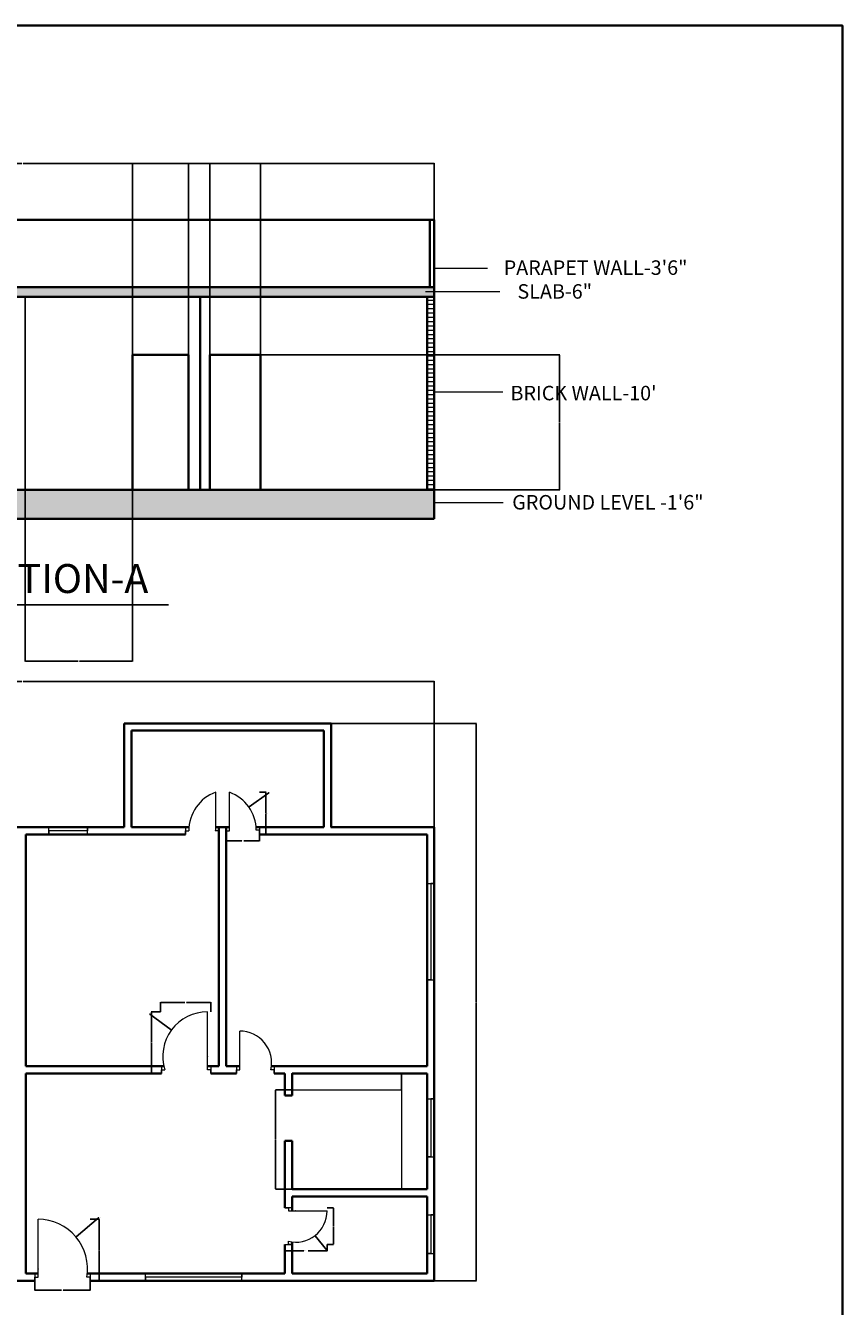
# Model space of a CAD drawing. Units: inches. Extents: x 2055 to 3558, y 1520 to 2888.
# Tile 8 of 8: x 3050 to 3558, y 2092 to 2888. Entities that reach past the tile are written whole.
import ezdxf

# ---------------------------------------------------------------- set-up
doc = ezdxf.new("R2010")
doc.units = ezdxf.units.IN
for name, color, linetype, lineweight in [('A-ANNO-DIMS', 2, 'Continuous', 18), ('A-ANNO-TEXT', 7, 'Continuous', 18), ('A-ANNO-TTLB', 7, 'Continuous', 35), ('A-DOOR', 3, 'Continuous', 18), ('A-FLOR-FIXT', 8, 'Continuous', 18), ('A-GLAZ', 4, 'Continuous', 18), ('A-SECT', 7, 'Continuous', 35), ('A-SECT-PATT', 252, 'Continuous', 13), ('A-WALL', 7, 'Continuous', 35), ('A-WALL-PATT', 252, 'Continuous', 13)]:
    doc.layers.add(name, color=color, linetype=linetype, lineweight=lineweight)
doc.styles.get("Standard").update_dxf_attribs({"font": 'arial.ttf'})
doc.dimstyles.get("Standard").update_dxf_attribs({"dimtxt": 0.18, "dimasz": 0.18, "dimexe": 0.18, "dimexo": 0.0625, "dimgap": 0.09, "dimtad": 0, "dimtih": 1, "dimtoh": 1, "dimdec": 4, "dimzin": 0, "dimdsep": 46, "dimtxsty": 'Standard', "dimcen": 0.09, "dimadec": 0, "dimazin": 0, "dimtfac": 1, "dimtdec": 4, "dimtofl": 0, "dimtmove": 0, "dimatfit": 3, "dimfxl": 1, "dimtolj": 1, "dimtzin": 0, "dimarcsym": 0})

# ---------------------------------------------------------------- blocks, each defined once
blk = doc.blocks.new('DOOR-BED-36-C')
for p, q in [((28.6, 2.25), (28.6, 38.25)), ((0, 4.5), (0, 0)), ((0, 0), (0, 2.25)), ((0, 2.25), (2, 2.25)), ((30.6, 2.25), (28.6, 2.25)), ((30.6, 4.5), (30.6, 0)), ((30.6, 0), (30.6, 2.25))]:
    blk.add_line(p, q)
blk.add_arc((28.6, 10.43), 27.83, 90, 197.08497)
blk = doc.blocks.new('DOOR-BED-24-A')
for p, q in [((2, 2.25), (2, 26.25)), ((0, 4.5), (0, 0)), ((0, 0), (0, 2.25)), ((0, 2.25), (2, 2.25)), ((23.39, 2.25), (21.39, 2.25)), ((23.39, 4.5), (23.39, 0)), ((23.39, 0), (23.39, 2.25))]:
    blk.add_line(p, q)
blk.add_arc((2, 6.42), 19.83, 347.8769, 90)
blk = doc.blocks.new('DOOR-BATH-24-A')
for p, q in [((4.5, 22.87), (0, 22.87)), ((0, 22.87), (2.25, 22.87)), ((2.25, 22.87), (2.25, 20.87)), ((2.25, 20.87), (26.25, 20.87)), ((2.25, 0), (2.25, 2)), ((0, 0), (4.5, 0)), ((4.5, 0), (2.25, 0))]:
    blk.add_line(p, q)
blk.add_arc((6.83, 20.87), 19.42, 256.35438, 0)
blk = doc.blocks.new('DOOR-ENTRY-36-A')
for p, q in [((2, 2.25), (2, 38.25)), ((0, 4.5), (0, 0)), ((0, 0), (0, 2.25)), ((0, 2.25), (2, 2.25)), ((34.35, 2.25), (32.35, 2.25)), ((34.35, 4.5), (34.35, 0)), ((34.35, 0), (34.35, 2.25))]:
    blk.add_line(p, q)
blk.add_arc((2, 7.46), 30.8, 350.26968, 90)
blk = doc.blocks.new('DOOR-VERANDA-24-G')
for p, q in [((18.74, 2.29), (18.74, 26.29)), ((0, 4.5), (0, 0)), ((0, 0), (0, 2.25)), ((0, 2.25), (2, 2.25)), ((20.74, 2.29), (18.74, 2.29))]:
    blk.add_line(p, q)
blk.add_arc((27.63, 2.25), 25.63, 110.29699, 180)
blk = doc.blocks.new('DOOR-VERANDA-24-H')
for p, q in [((2, 2.19), (2, 26.19)), ((0, 2.19), (2, 2.19)), ((20.78, 2.69), (18.78, 2.69)), ((20.78, 4.5), (20.78, 0)), ((20.78, 0), (20.78, 2.69))]:
    blk.add_line(p, q)
blk.add_arc((-6.63, 2.38), 25.41, 0.68308, 70.14714)
blk = doc.blocks.new('WIN-36')
for p, q in [((2.25, 36), (0, 36)), ((0, 36), (4.5, 36)), ((2.25, 0), (2.25, 36)), ((0, 0), (4.5, 0)), ((4.5, 0), (2.25, 0))]:
    blk.add_line(p, q)
blk = doc.blocks.new('WIN-24')
for p, q in [((0, 24), (4.5, 24)), ((4.5, 24), (2.25, 24)), ((2.25, 24), (2.25, 0)), ((2.25, 0), (0, 0)), ((0, 0), (4.5, 0))]:
    blk.add_line(p, q)
blk = doc.blocks.new('WIN-60')
for p, q in [((0, 60), (4.5, 60)), ((4.5, 60), (2.25, 60)), ((2.25, 60), (2.25, 0)), ((2.25, 0), (0, 0)), ((0, 0), (4.5, 0))]:
    blk.add_line(p, q)
blk = doc.blocks.new('COUNTER-2')
for p, q in [((0, 61.79), (68.13, 61.79)), ((68.13, 61.79), (68.13, 0))]:
    blk.add_line(p, q)
blk = doc.blocks.new('VERANDA-PERIMETER')
for p, q in [((0, 0), (0, 64.5)), ((4.5, 64.5), (4.5, 4.5)), ((124.15, 4.5), (124.15, 64.5)), ((128.65, 64.5), (128.65, 4.5)), ((4.5, 0), (0, 0)), ((4.5, 4.5), (124.15, 4.5)), ((128.65, 0), (4.5, 0)), ((128.65, 4.5), (128.65, 0))]:
    blk.add_line(p, q)
blk = doc.blocks.new('*D56')
at = {"layer": 'A-ANNO-DIMS', "color": 0, "lineweight": -2, "transparency": 16777216}
for p, q in [((3133.65, 2275.25), (3127.79, 2275.25)), ((3127.97, 2275.07), (3127.97, 2256.31)), ((3127.97, 2237.18), (3127.97, 2255.94)), ((3133.65, 2237), (3127.79, 2237))]:
    blk.add_line(p, q, dxfattribs=at)
at = {"layer": 'A-ANNO-DIMS', "color": 0, "transparency": 16777216}
for points in [[(3127.94, 2275.07), (3128, 2275.07), (3127.97, 2275.25)], [(3127.94, 2237.18), (3128, 2237.18), (3127.97, 2237)]]:
    blk.add_solid(points, dxfattribs=at)
at = {"layer": 'Defpoints', "color": 0, "transparency": 16777216}
for p in [(3127.97, 2275.25), (3133.71, 2275.25), (3133.71, 2237)]:
    blk.add_point(p, dxfattribs=at)
at = {"layer": 'A-ANNO-DIMS', "color": 0, "transparency": 16777216, "insert": (3127.97, 2256.12), "char_height": 0.18, "attachment_point": 5}
blk.add_mtext('\\A1;BED DOOR 38 TYP.', dxfattribs=at)
blk = doc.blocks.new('*D57')
at = {"layer": 'A-ANNO-DIMS', "color": 0, "lineweight": -2, "transparency": 16777216}
for p, q in [((3133.71, 2275.31), (3133.71, 2281.17)), ((3133.89, 2280.99), (3148.78, 2280.99)), ((3164.72, 2280.99), (3149.83, 2280.99)), ((3164.9, 2275.31), (3164.9, 2281.17))]:
    blk.add_line(p, q, dxfattribs=at)
at = {"layer": 'A-ANNO-DIMS', "color": 0, "transparency": 16777216}
for points in [[(3133.89, 2281.02), (3133.89, 2280.96), (3133.71, 2280.99)], [(3164.72, 2281.02), (3164.72, 2280.96), (3164.9, 2280.99)]]:
    blk.add_solid(points, dxfattribs=at)
at = {"layer": 'Defpoints', "color": 0, "transparency": 16777216}
for p in [(3164.9, 2280.99), (3133.71, 2275.25), (3164.9, 2275.25)]:
    blk.add_point(p, dxfattribs=at)
at = {"layer": 'A-ANNO-DIMS', "color": 0, "transparency": 16777216, "insert": (3149.3, 2280.99), "char_height": 0.18, "attachment_point": 5}
blk.add_mtext('\\A1;31 TYP.', dxfattribs=at)
blk = doc.blocks.new('*D60')
at = {"layer": 'A-ANNO-DIMS', "color": 0, "lineweight": -2, "transparency": 16777216}
for p, q in [((3211, 2130.52), (3211, 2126.46)), ((3211.18, 2126.64), (3222.81, 2126.64)), ((3237.07, 2126.64), (3225.43, 2126.64)), ((3237.25, 2130.52), (3237.25, 2126.46))]:
    blk.add_line(p, q, dxfattribs=at)
at = {"layer": 'A-ANNO-DIMS', "color": 0, "transparency": 16777216}
for points in [[(3211.18, 2126.67), (3211.18, 2126.61), (3211, 2126.64)], [(3237.07, 2126.67), (3237.07, 2126.61), (3237.25, 2126.64)]]:
    blk.add_solid(points, dxfattribs=at)
at = {"layer": 'Defpoints', "color": 0, "transparency": 16777216}
for p in [(3211, 2130.58), (3237.25, 2130.58), (3237.25, 2126.64)]:
    blk.add_point(p, dxfattribs=at)
at = {"layer": 'A-ANNO-DIMS', "color": 0, "transparency": 16777216, "insert": (3224.12, 2126.64), "char_height": 0.18, "attachment_point": 5}
blk.add_mtext('\\A1;BATH DOOR 26 TYP.', dxfattribs=at)
blk = doc.blocks.new('*D61')
at = {"layer": 'A-ANNO-DIMS', "color": 0, "lineweight": -2, "transparency": 16777216}
for p, q in [((3237.31, 2153.45), (3241.36, 2153.45)), ((3241.18, 2153.27), (3241.18, 2142.2)), ((3241.18, 2130.76), (3241.18, 2141.84)), ((3237.31, 2130.58), (3241.36, 2130.58))]:
    blk.add_line(p, q, dxfattribs=at)
at = {"layer": 'A-ANNO-DIMS', "color": 0, "transparency": 16777216}
for points in [[(3241.15, 2153.27), (3241.21, 2153.27), (3241.18, 2153.45)], [(3241.15, 2130.76), (3241.21, 2130.76), (3241.18, 2130.58)]]:
    blk.add_solid(points, dxfattribs=at)
at = {"layer": 'Defpoints', "color": 0, "transparency": 16777216}
for p in [(3237.25, 2153.45), (3241.18, 2153.45), (3237.25, 2130.58)]:
    blk.add_point(p, dxfattribs=at)
at = {"layer": 'A-ANNO-DIMS', "color": 0, "transparency": 16777216, "insert": (3241.18, 2142.02), "char_height": 0.18, "attachment_point": 5}
blk.add_mtext('\\A1;23 TYP.', dxfattribs=at)
blk = doc.blocks.new('*D62')
at = {"layer": 'A-ANNO-DIMS', "color": 0, "lineweight": -2, "transparency": 16777216}
for p, q in [((3089.92, 2146.25), (3095.78, 2146.25)), ((3095.6, 2146.07), (3095.6, 2127.31)), ((3095.6, 2108.18), (3095.6, 2126.94)), ((3089.92, 2108), (3095.78, 2108))]:
    blk.add_line(p, q, dxfattribs=at)
at = {"layer": 'A-ANNO-DIMS', "color": 0, "transparency": 16777216}
for points in [[(3095.57, 2146.07), (3095.63, 2146.07), (3095.6, 2146.25)], [(3095.57, 2108.18), (3095.63, 2108.18), (3095.6, 2108)]]:
    blk.add_solid(points, dxfattribs=at)
at = {"layer": 'Defpoints', "color": 0, "transparency": 16777216}
for p in [(3089.86, 2146.25), (3095.6, 2146.25), (3089.86, 2108)]:
    blk.add_point(p, dxfattribs=at)
at = {"layer": 'A-ANNO-DIMS', "color": 0, "transparency": 16777216, "insert": (3095.6, 2127.12), "char_height": 0.18, "attachment_point": 5}
blk.add_mtext('\\A1;ENTRY DOOR 38 TYP.', dxfattribs=at)
blk = doc.blocks.new('*D63')
at = {"layer": 'A-ANNO-DIMS', "color": 0, "lineweight": -2, "transparency": 16777216}
for p, q in [((3055.51, 2107.94), (3055.51, 2102.08)), ((3055.69, 2102.26), (3072.16, 2102.26)), ((3089.68, 2102.26), (3073.21, 2102.26)), ((3089.86, 2107.94), (3089.86, 2102.08))]:
    blk.add_line(p, q, dxfattribs=at)
at = {"layer": 'A-ANNO-DIMS', "color": 0, "transparency": 16777216}
for points in [[(3055.69, 2102.29), (3055.69, 2102.23), (3055.51, 2102.26)], [(3089.68, 2102.29), (3089.68, 2102.23), (3089.86, 2102.26)]]:
    blk.add_solid(points, dxfattribs=at)
at = {"layer": 'Defpoints', "color": 0, "transparency": 16777216}
for p in [(3055.51, 2108), (3089.86, 2108), (3089.86, 2102.26)]:
    blk.add_point(p, dxfattribs=at)
at = {"layer": 'A-ANNO-DIMS', "color": 0, "transparency": 16777216, "insert": (3072.69, 2102.26), "char_height": 0.18, "attachment_point": 5}
blk.add_mtext('\\A1;34 TYP.', dxfattribs=at)
blk = doc.blocks.new('*D96')
at = {"layer": 'A-ANNO-DIMS', "color": 0, "lineweight": -2, "transparency": 16777216}
for p, q in [((3195.34, 2411.79), (3199.4, 2411.79)), ((3199.22, 2411.61), (3199.22, 2398.83)), ((3199.22, 2385.68), (3199.22, 2398.46)), ((3195.34, 2385.5), (3199.4, 2385.5))]:
    blk.add_line(p, q, dxfattribs=at)
at = {"layer": 'A-ANNO-DIMS', "color": 0, "transparency": 16777216}
for points in [[(3199.19, 2411.61), (3199.25, 2411.61), (3199.22, 2411.79)], [(3199.19, 2385.68), (3199.25, 2385.68), (3199.22, 2385.5)]]:
    blk.add_solid(points, dxfattribs=at)
at = {"layer": 'Defpoints', "color": 0, "transparency": 16777216}
for p in [(3195.28, 2411.79), (3199.22, 2411.79), (3195.28, 2385.5)]:
    blk.add_point(p, dxfattribs=at)
at = {"layer": 'A-ANNO-DIMS', "color": 0, "transparency": 16777216, "insert": (3199.22, 2398.64), "char_height": 0.18, "attachment_point": 5}
blk.add_mtext('\\A1;VERANDA DOOR 26 TYP.', dxfattribs=at)
blk = doc.blocks.new('*D97')
at = {"layer": 'A-ANNO-DIMS', "color": 0, "lineweight": -2, "transparency": 16777216}
for p, q in [((3174.5, 2385.44), (3174.5, 2381.38)), ((3174.68, 2381.56), (3184.36, 2381.56)), ((3195.1, 2381.56), (3185.42, 2381.56)), ((3195.28, 2385.44), (3195.28, 2381.38))]:
    blk.add_line(p, q, dxfattribs=at)
at = {"layer": 'A-ANNO-DIMS', "color": 0, "transparency": 16777216}
for points in [[(3174.68, 2381.59), (3174.68, 2381.53), (3174.5, 2381.56)], [(3195.1, 2381.59), (3195.1, 2381.53), (3195.28, 2381.56)]]:
    blk.add_solid(points, dxfattribs=at)
at = {"layer": 'Defpoints', "color": 0, "transparency": 16777216}
for p in [(3174.5, 2385.5), (3195.28, 2385.5), (3195.28, 2381.56)]:
    blk.add_point(p, dxfattribs=at)
at = {"layer": 'A-ANNO-DIMS', "color": 0, "transparency": 16777216, "insert": (3184.89, 2381.56), "char_height": 0.18, "attachment_point": 5}
blk.add_mtext('\\A1;21 TYP.', dxfattribs=at)
blk = doc.blocks.new('*D108')
at = {"layer": 'A-ANNO-DIMS', "color": 0, "lineweight": -2, "transparency": 16777216}
for p, q in [((3215.5, 2226.85), (3215.5, 2237.19)), ((3283.62, 2226.85), (3283.62, 2237.19)), ((3215.68, 2237.01), (3248.38, 2237.01)), ((3283.44, 2237.01), (3250.74, 2237.01))]:
    blk.add_line(p, q, dxfattribs=at)
at = {"layer": 'A-ANNO-DIMS', "color": 0, "transparency": 16777216}
for points in [[(3215.68, 2237.04), (3215.68, 2236.98), (3215.5, 2237.01)], [(3283.44, 2237.04), (3283.44, 2236.98), (3283.62, 2237.01)]]:
    blk.add_solid(points, dxfattribs=at)
at = {"layer": 'Defpoints', "color": 0, "transparency": 16777216}
for p in [(3283.62, 2237.01), (3215.5, 2226.79), (3283.62, 2226.79)]:
    blk.add_point(p, dxfattribs=at)
at = {"layer": 'A-ANNO-DIMS', "color": 0, "transparency": 16777216, "insert": (3249.56, 2237.01), "char_height": 0.18, "attachment_point": 5}
blk.add_mtext('\\A1;COUNTER 68 TYP.', dxfattribs=at)
blk = doc.blocks.new('*D109')
at = {"layer": 'A-ANNO-DIMS', "color": 0, "lineweight": -2, "transparency": 16777216}
for p, q in [((3215.43, 2226.79), (3205.1, 2226.79)), ((3205.28, 2226.61), (3205.28, 2196.08)), ((3205.28, 2165.18), (3205.28, 2195.71)), ((3215.43, 2165), (3205.1, 2165))]:
    blk.add_line(p, q, dxfattribs=at)
at = {"layer": 'A-ANNO-DIMS', "color": 0, "transparency": 16777216}
for points in [[(3205.25, 2226.61), (3205.31, 2226.61), (3205.28, 2226.79)], [(3205.25, 2165.18), (3205.31, 2165.18), (3205.28, 2165)]]:
    blk.add_solid(points, dxfattribs=at)
at = {"layer": 'Defpoints', "color": 0, "transparency": 16777216}
for p in [(3205.28, 2226.79), (3215.5, 2226.79), (3215.5, 2165)]:
    blk.add_point(p, dxfattribs=at)
at = {"layer": 'A-ANNO-DIMS', "color": 0, "transparency": 16777216, "insert": (3205.28, 2195.9), "char_height": 0.18, "attachment_point": 5}
blk.add_mtext('\\A1;62 TYP.', dxfattribs=at)
blk = doc.blocks.new('*D124')
at = {"layer": 'A-ANNO-DIMS', "color": 0, "lineweight": -2, "transparency": 16777216}
for p, q in [((2791.5, 2390.06), (2791.5, 2480.78)), ((2791.68, 2480.6), (3047.35, 2480.6)), ((3303.82, 2480.6), (3048.14, 2480.6)), ((3304, 2390.06), (3304, 2480.78))]:
    blk.add_line(p, q, dxfattribs=at)
at = {"layer": 'A-ANNO-DIMS', "color": 0, "transparency": 16777216}
for points in [[(2791.68, 2480.63), (2791.68, 2480.57), (2791.5, 2480.6)], [(3303.82, 2480.63), (3303.82, 2480.57), (3304, 2480.6)]]:
    blk.add_solid(points, dxfattribs=at)
at = {"layer": 'Defpoints', "color": 0, "transparency": 16777216}
for p in [(3304, 2480.6), (2791.5, 2390), (3304, 2390)]:
    blk.add_point(p, dxfattribs=at)
at = {"layer": 'A-ANNO-DIMS', "color": 0, "transparency": 16777216, "insert": (3047.75, 2480.6), "char_height": 0.18, "attachment_point": 5}
blk.add_mtext('\\A1;512.5', dxfattribs=at)
blk = doc.blocks.new('*D125')
at = {"layer": 'A-ANNO-DIMS', "color": 0, "lineweight": -2, "transparency": 16777216}
for p, q in [((3239.79, 2454.5), (3330.28, 2454.5)), ((3330.1, 2454.32), (3330.1, 2281.43)), ((3330.1, 2108.18), (3330.1, 2281.07)), ((3304.06, 2108), (3330.28, 2108))]:
    blk.add_line(p, q, dxfattribs=at)
at = {"layer": 'A-ANNO-DIMS', "color": 0, "transparency": 16777216}
for points in [[(3330.07, 2454.32), (3330.13, 2454.32), (3330.1, 2454.5)], [(3330.07, 2108.18), (3330.13, 2108.18), (3330.1, 2108)]]:
    blk.add_solid(points, dxfattribs=at)
at = {"layer": 'Defpoints', "color": 0, "transparency": 16777216}
for p in [(3239.72, 2454.5), (3330.1, 2454.5), (3304, 2108)]:
    blk.add_point(p, dxfattribs=at)
at = {"layer": 'A-ANNO-DIMS', "color": 0, "transparency": 16777216, "insert": (3330.1, 2281.25), "char_height": 0.18, "attachment_point": 5}
blk.add_mtext('\\A1;346.5', dxfattribs=at)
blk = doc.blocks.new('*D149')
at = {"layer": 'A-ANNO-DIMS', "color": 0, "lineweight": -2, "transparency": 16777216}
for p, q in [((2791.5, 2767.66), (2791.5, 2802.68)), ((2791.68, 2802.5), (3047.35, 2802.5)), ((3303.82, 2802.5), (3048.14, 2802.5)), ((3304, 2767.66), (3304, 2802.68))]:
    blk.add_line(p, q, dxfattribs=at)
at = {"layer": 'A-ANNO-DIMS', "color": 0, "transparency": 16777216}
for points in [[(2791.68, 2802.53), (2791.68, 2802.47), (2791.5, 2802.5)], [(3303.82, 2802.53), (3303.82, 2802.47), (3304, 2802.5)]]:
    blk.add_solid(points, dxfattribs=at)
at = {"layer": 'Defpoints', "color": 0, "transparency": 16777216}
for p in [(3304, 2802.5), (2791.5, 2767.6), (3304, 2767.6)]:
    blk.add_point(p, dxfattribs=at)
at = {"layer": 'A-ANNO-DIMS', "color": 0, "transparency": 16777216, "insert": (3047.75, 2802.5), "char_height": 0.18, "attachment_point": 5}
blk.add_mtext('\\A1;512.5', dxfattribs=at)
blk = doc.blocks.new('*D153')
at = {"layer": 'A-ANNO-DIMS', "color": 0, "lineweight": -2, "transparency": 16777216}
for p, q in [((3049.5, 2719.54), (3049.5, 2493.05)), ((3116.25, 2683.54), (3116.25, 2493.05)), ((3049.68, 2493.23), (3082.48, 2493.23)), ((3116.07, 2493.23), (3083.27, 2493.23))]:
    blk.add_line(p, q, dxfattribs=at)
at = {"layer": 'A-ANNO-DIMS', "color": 0, "transparency": 16777216}
for points in [[(3049.68, 2493.26), (3049.68, 2493.2), (3049.5, 2493.23)], [(3116.07, 2493.26), (3116.07, 2493.2), (3116.25, 2493.23)]]:
    blk.add_solid(points, dxfattribs=at)
at = {"layer": 'Defpoints', "color": 0, "transparency": 16777216}
for p in [(3049.5, 2719.6), (3116.25, 2683.6), (3116.25, 2493.23)]:
    blk.add_point(p, dxfattribs=at)
at = {"layer": 'A-ANNO-DIMS', "color": 0, "transparency": 16777216, "insert": (3082.87, 2493.23), "char_height": 0.18, "attachment_point": 5}
blk.add_mtext('\\A1;66.76', dxfattribs=at)
blk = doc.blocks.new('*D157')
at = {"layer": 'A-ANNO-DIMS', "color": 0, "lineweight": -2, "transparency": 16777216}
for p, q in [((3116.25, 2683.66), (3116.25, 2802.68)), ((3116.43, 2802.5), (3133.23, 2802.5)), ((3150.96, 2802.5), (3134.16, 2802.5)), ((3151.14, 2683.66), (3151.14, 2802.68))]:
    blk.add_line(p, q, dxfattribs=at)
at = {"layer": 'A-ANNO-DIMS', "color": 0, "transparency": 16777216}
for points in [[(3116.43, 2802.53), (3116.43, 2802.47), (3116.25, 2802.5)], [(3150.96, 2802.53), (3150.96, 2802.47), (3151.14, 2802.5)]]:
    blk.add_solid(points, dxfattribs=at)
at = {"layer": 'Defpoints', "color": 0, "transparency": 16777216}
for p in [(3151.14, 2802.5), (3116.25, 2683.6), (3151.14, 2683.6)]:
    blk.add_point(p, dxfattribs=at)
at = {"layer": 'A-ANNO-DIMS', "color": 0, "transparency": 16777216, "insert": (3133.7, 2802.5), "char_height": 0.18, "attachment_point": 5}
blk.add_mtext('\\A1;34.885', dxfattribs=at)
blk = doc.blocks.new('*D158')
at = {"layer": 'A-ANNO-DIMS', "color": 0, "lineweight": -2, "transparency": 16777216}
for p, q in [((3151.14, 2683.66), (3151.14, 2802.68)), ((3151.32, 2802.5), (3157.27, 2802.5)), ((3164.12, 2802.5), (3158.18, 2802.5)), ((3164.3, 2683.66), (3164.3, 2802.68))]:
    blk.add_line(p, q, dxfattribs=at)
at = {"layer": 'A-ANNO-DIMS', "color": 0, "transparency": 16777216}
for points in [[(3151.32, 2802.53), (3151.32, 2802.47), (3151.14, 2802.5)], [(3164.12, 2802.53), (3164.12, 2802.47), (3164.3, 2802.5)]]:
    blk.add_solid(points, dxfattribs=at)
at = {"layer": 'Defpoints', "color": 0, "transparency": 16777216}
for p in [(3164.3, 2802.5), (3151.14, 2683.6), (3164.3, 2683.6)]:
    blk.add_point(p, dxfattribs=at)
at = {"layer": 'A-ANNO-DIMS', "color": 0, "transparency": 16777216, "insert": (3157.72, 2802.5), "char_height": 0.18, "attachment_point": 5}
blk.add_mtext('\\A1;13.164', dxfattribs=at)
blk = doc.blocks.new('*D159')
at = {"layer": 'A-ANNO-DIMS', "color": 0, "lineweight": -2, "transparency": 16777216}
for p, q in [((3164.3, 2683.66), (3164.3, 2802.68)), ((3164.48, 2802.5), (3179.69, 2802.5)), ((3195.69, 2802.5), (3180.48, 2802.5)), ((3195.87, 2683.66), (3195.87, 2802.68))]:
    blk.add_line(p, q, dxfattribs=at)
at = {"layer": 'A-ANNO-DIMS', "color": 0, "transparency": 16777216}
for points in [[(3164.48, 2802.53), (3164.48, 2802.47), (3164.3, 2802.5)], [(3195.69, 2802.53), (3195.69, 2802.47), (3195.87, 2802.5)]]:
    blk.add_solid(points, dxfattribs=at)
at = {"layer": 'Defpoints', "color": 0, "transparency": 16777216}
for p in [(3195.87, 2802.5), (3164.3, 2683.6), (3195.87, 2683.6)]:
    blk.add_point(p, dxfattribs=at)
at = {"layer": 'A-ANNO-DIMS', "color": 0, "transparency": 16777216, "insert": (3180.09, 2802.5), "char_height": 0.18, "attachment_point": 5}
blk.add_mtext('\\A1;31.57', dxfattribs=at)
blk = doc.blocks.new('*D160')
at = {"layer": 'A-ANNO-DIMS', "color": 0, "lineweight": -2, "transparency": 16777216}
for p, q in [((3195.93, 2683.6), (3382, 2683.6)), ((3381.82, 2683.42), (3381.82, 2641.78)), ((3381.82, 2599.78), (3381.82, 2641.42)), ((3195.93, 2599.6), (3382, 2599.6))]:
    blk.add_line(p, q, dxfattribs=at)
at = {"layer": 'A-ANNO-DIMS', "color": 0, "transparency": 16777216}
for points in [[(3381.79, 2683.42), (3381.85, 2683.42), (3381.82, 2683.6)], [(3381.79, 2599.78), (3381.85, 2599.78), (3381.82, 2599.6)]]:
    blk.add_solid(points, dxfattribs=at)
at = {"layer": 'Defpoints', "color": 0, "transparency": 16777216}
for p in [(3195.87, 2683.6), (3381.82, 2683.6), (3195.87, 2599.6)]:
    blk.add_point(p, dxfattribs=at)
at = {"layer": 'A-ANNO-DIMS', "color": 0, "transparency": 16777216, "insert": (3381.82, 2641.6), "char_height": 0.18, "attachment_point": 5}
blk.add_mtext('\\A1;84', dxfattribs=at)
blk = doc.blocks.new('*D162')
at = {"layer": 'A-ANNO-DIMS', "color": 0, "lineweight": -2, "transparency": 16777216}
for p, q in [((3095.18, 2147.21), (3081.19, 2135.42)), ((3095.36, 2147.21), (3095.18, 2147.21)), ((3057.42, 2115.45), (3057.6, 2115.45)), ((3057.51, 2115.36), (3057.51, 2115.54))]:
    blk.add_line(p, q, dxfattribs=at)
at = {"layer": 'A-ANNO-DIMS', "color": 0, "transparency": 16777216}
blk.add_solid([(3081.17, 2135.44), (3081.21, 2135.4), (3081.05, 2135.3)], dxfattribs=at)
at = {"layer": 'Defpoints', "color": 0, "transparency": 16777216}
for p in [(3081.05, 2135.3), (3057.51, 2115.45)]:
    blk.add_point(p, dxfattribs=at)
at = {"layer": 'A-ANNO-DIMS', "color": 0, "transparency": 16777216, "insert": (3095.91, 2147.21), "char_height": 0.18, "attachment_point": 5}
blk.add_mtext('\\A1;R30.795', dxfattribs=at)
blk = doc.blocks.new('*D163')
at = {"layer": 'A-ANNO-DIMS', "color": 0, "lineweight": -2, "transparency": 16777216}
for p, q in [((3126.91, 2273.88), (3127.09, 2273.88)), ((3127.09, 2273.88), (3140.38, 2264.07)), ((3162.81, 2247.42), (3162.99, 2247.42)), ((3162.9, 2247.33), (3162.9, 2247.51))]:
    blk.add_line(p, q, dxfattribs=at)
at = {"layer": 'A-ANNO-DIMS', "color": 0, "transparency": 16777216}
blk.add_solid([(3140.39, 2264.09), (3140.36, 2264.04), (3140.52, 2263.96)], dxfattribs=at)
at = {"layer": 'Defpoints', "color": 0, "transparency": 16777216}
for p in [(3140.52, 2263.96), (3162.9, 2247.42)]:
    blk.add_point(p, dxfattribs=at)
at = {"layer": 'A-ANNO-DIMS', "color": 0, "transparency": 16777216, "insert": (3126.36, 2273.88), "char_height": 0.18, "attachment_point": 5}
blk.add_mtext('\\A1;R27.825', dxfattribs=at)
blk = doc.blocks.new('*D167')
at = {"layer": 'A-ANNO-DIMS', "color": 0, "lineweight": -2, "transparency": 16777216}
for p, q in [((3201, 2411.45), (3188.72, 2402.71)), ((3201.18, 2411.45), (3201, 2411.45)), ((3167.77, 2387.88), (3167.95, 2387.88)), ((3167.86, 2387.79), (3167.86, 2387.97))]:
    blk.add_line(p, q, dxfattribs=at)
at = {"layer": 'A-ANNO-DIMS', "color": 0, "transparency": 16777216}
blk.add_solid([(3188.71, 2402.74), (3188.74, 2402.69), (3188.58, 2402.61)], dxfattribs=at)
at = {"layer": 'Defpoints', "color": 0, "transparency": 16777216}
for p in [(3188.58, 2402.61), (3167.86, 2387.88)]:
    blk.add_point(p, dxfattribs=at)
at = {"layer": 'A-ANNO-DIMS', "color": 0, "transparency": 16777216, "insert": (3201.73, 2411.45), "char_height": 0.18, "attachment_point": 5}
blk.add_mtext('\\A1;R25.414', dxfattribs=at)
blk = doc.blocks.new('*D169')
at = {"layer": 'A-ANNO-DIMS', "color": 0, "lineweight": -2, "transparency": 16777216}
for p, q in [((3217.74, 2151.45), (3217.92, 2151.45)), ((3217.83, 2151.36), (3217.83, 2151.54)), ((3237.03, 2127.03), (3229.94, 2136.05)), ((3237.21, 2127.03), (3237.03, 2127.03))]:
    blk.add_line(p, q, dxfattribs=at)
at = {"layer": 'A-ANNO-DIMS', "color": 0, "transparency": 16777216}
blk.add_solid([(3229.96, 2136.06), (3229.92, 2136.03), (3229.83, 2136.19)], dxfattribs=at)
at = {"layer": 'Defpoints', "color": 0, "transparency": 16777216}
for p in [(3217.83, 2151.45), (3229.83, 2136.19)]:
    blk.add_point(p, dxfattribs=at)
at = {"layer": 'A-ANNO-DIMS', "color": 0, "transparency": 16777216, "insert": (3237.69, 2127.03), "char_height": 0.18, "attachment_point": 5}
blk.add_mtext('\\A1;R19.42', dxfattribs=at)

msp = doc.modelspace()

# ---------------------------------------------------------------- hatches: boundary and pattern name
at = {"layer": 'A-SECT-PATT'}
h = msp.add_hatch(dxfattribs=at)
h.set_pattern_fill('AR-CONC', color=256, scale=0.0531496, style=0)
h.paths.add_polyline_path([(2791.4955, 2719.5987), (3303.9955, 2719.5987), (3303.9955, 2725.5987), (2791.4955, 2725.5987)])
h = msp.add_hatch(dxfattribs=at)
h.set_pattern_fill('AR-CONC', color=256, scale=0.07874016, style=0)
h.paths.add_polyline_path([(2791.4955, 2581.5987), (3303.9955, 2581.5987), (3303.9955, 2599.5987), (2791.4955, 2599.5987)])
at = {"layer": 'A-WALL-PATT'}
h = msp.add_hatch(dxfattribs=at)
h.set_pattern_fill('AR-BRSTD', color=256, scale=0.03937008, style=0)
h.paths.add_polyline_path([(3299.4955, 2599.5987), (3303.9955, 2599.5987), (3303.9955, 2719.5987), (3299.4955, 2719.5987)])

# ---------------------------------------------------------------- linework, layer by layer
at = {"layer": 'A-ANNO-TEXT'}
for p, q in [((3303.9955, 2737.4345), (3337.0022, 2737.4345)), ((3298.5436, 2722.9693), (3344.7116, 2722.9693)), ((3303.9955, 2660.6572), (3346.6825, 2660.6572)), ((3303.9955, 2591.9051), (3346.9218, 2591.9051)), ((3138.6573, 2528.1346), (2995.5972, 2528.1346)), ((3002.7098, 2528.1346), (3138.6573, 2528.1346))]:
    msp.add_line(p, q, dxfattribs=at)
at = {"layer": 'A-ANNO-TTLB'}
msp.add_lwpolyline([(2054.7598, 2888.2545), (3557.8479, 2888.2545), (3557.8479, 1520.3256), (2054.7598, 1520.3256)], close=True, dxfattribs=at)
at = {"layer": 'A-SECT'}
for p, q in [((3303.9955, 2767.5987), (2791.4955, 2767.5987)), ((3301.2266, 2725.5987), (3301.2266, 2767.5987)), ((3303.9955, 2767.5987), (3303.9955, 2581.5987)), ((3303.9955, 2725.5987), (2791.4955, 2725.5987)), ((3303.9955, 2719.5987), (2791.4955, 2719.5987)), ((3158.3736, 2599.5987), (3158.3736, 2719.5987)), ((3299.4955, 2719.5987), (3299.4955, 2599.5987)), ((3116.2543, 2683.5987), (3116.2543, 2599.5987)), ((3151.1389, 2683.5987), (3116.2543, 2683.5987)), ((3151.1389, 2683.5987), (3151.1389, 2599.5987)), ((3164.3033, 2683.5987), (3164.3033, 2599.5987)), ((3195.8714, 2683.5987), (3164.3033, 2683.5987)), ((3195.8714, 2683.5987), (3195.8714, 2599.5987)), ((3303.9955, 2599.5987), (2791.4955, 2599.5987)), ((3303.9955, 2581.5987), (2791.4955, 2581.5987))]:
    msp.add_line(p, q, dxfattribs=at)
at = {"layer": 'A-WALL'}
for p, q in [((2981.9137, 2389.9995), (3111.0777, 2389.9995)), ((2981.9137, 2389.9995), (3111.0777, 2389.9995)), ((3115.5777, 2389.9995), (3151.3565, 2389.9995)), ((3115.5777, 2389.9995), (3151.3565, 2389.9995)), ((3167.9955, 2389.9995), (3176.4955, 2389.9995)), ((3167.9955, 2389.9995), (3176.4955, 2389.9995)), ((3169.9955, 2389.9995), (3169.9955, 2241.4995)), ((3174.4955, 2389.9995), (3174.4955, 2241.4995)), ((3193.1906, 2389.9995), (3235.2239, 2389.9995)), ((3193.1906, 2389.9995), (3235.2239, 2389.9995)), ((3239.7239, 2389.9995), (3303.9955, 2389.9995)), ((3239.7239, 2389.9995), (3303.9955, 2389.9995)), ((3303.9955, 2389.9995), (3303.9955, 2107.9995)), ((3049.9955, 2385.4995), (3149.2575, 2385.4995)), ((3049.9955, 2385.4995), (3049.9955, 2241.4995)), ((3195.2772, 2385.4995), (3299.4955, 2385.4995)), ((3299.4955, 2385.4995), (3299.4955, 2241.4995)), ((3049.9955, 2241.4995), (3135.7132, 2241.4995)), ((3162.9003, 2241.4995), (3169.9955, 2241.4995)), ((3174.4955, 2241.4995), (3182.934, 2241.4995)), ((3202.6758, 2241.4995), (3299.4955, 2241.4995)), ((3215.4955, 2241.4995), (3210.9955, 2241.4995)), ((3049.9955, 2236.9995), (3134.303, 2236.9995)), ((3049.9955, 2236.9995), (3049.9955, 2112.4995)), ((3164.9003, 2236.9995), (3180.934, 2236.9995)), ((3204.3262, 2236.9995), (3210.9955, 2236.9995)), ((3210.9955, 2236.9995), (3210.9955, 2223.192)), ((3215.4955, 2236.9995), (3299.4955, 2236.9995)), ((3215.4955, 2223.192), (3215.4955, 2236.9995)), ((3299.4955, 2236.9995), (3299.4955, 2164.9995)), ((3210.9955, 2223.192), (3215.4955, 2223.192)), ((3210.9955, 2194.9685), (3210.9955, 2153.4523)), ((3215.4955, 2194.9685), (3210.9955, 2194.9685)), ((3215.4955, 2164.9995), (3215.4955, 2194.9685)), ((3215.4955, 2164.9995), (3299.4955, 2164.9995)), ((3215.4955, 2160.4995), (3299.4955, 2160.4995)), ((3215.4955, 2151.4523), (3215.4955, 2160.4995)), ((3299.4955, 2160.4995), (3299.4955, 2112.4995)), ((3210.9955, 2130.5817), (3210.9955, 2112.4995)), ((3215.4955, 2112.4995), (3215.4955, 2132.174)), ((3049.9955, 2112.4995), (3057.5099, 2112.4995)), ((3088.163, 2112.4995), (3210.9955, 2112.4995)), ((3215.4955, 2112.4995), (3299.4955, 2112.4995)), ((3039.1791, 2107.9995), (3055.5099, 2107.9995)), ((3089.8621, 2107.9995), (3303.9955, 2107.9995)), ((3299.4955, 2107.9995), (3215.4955, 2107.9995))]:
    msp.add_line(p, q, dxfattribs=at)

# ---------------------------------------------------------------- block references
at = {"layer": 'A-DOOR'}
for name, p in [('DOOR-VERANDA-24-G', (3149.2578, 2385.499)), ('DOOR-VERANDA-24-H', (3174.4958, 2385.499)), ('DOOR-BED-36-C', (3134.3028, 2236.999)), ('DOOR-BED-24-A', (3180.9338, 2236.999)), ('DOOR-BATH-24-A', (3210.9958, 2130.582)), ('DOOR-ENTRY-36-A', (3055.5098, 2107.999))]:
    msp.add_blockref(name, p, dxfattribs=at)
at = {"layer": 'A-FLOR-FIXT'}
msp.add_blockref('COUNTER-2', (3215.4958, 2164.999), dxfattribs=at)
at = {"layer": 'A-GLAZ', "extrusion": (0, 0, -1), "zscale": -1}
for name, p, rotation in [('WIN-24', (-3064.2815, 2385.4998), 90), ('WIN-36', (-3299.4958, 2221.1923), 180), ('WIN-60', (-3124.2386, 2107.9998), 90)]:
    msp.add_blockref(name, p, dxfattribs=dict(at, rotation=rotation))
at = {"layer": 'A-GLAZ'}
for name, p in [('WIN-60', (3299.4958, 2295.066)), ('WIN-24', (3299.4958, 2125.0333))]:
    msp.add_blockref(name, p, dxfattribs=at)
at = {"layer": 'A-WALL', "extrusion": (0, 0, -1), "zscale": -1, "rotation": 180}
msp.add_blockref('VERANDA-PERIMETER', (-3111.0777, 2454.5), dxfattribs=at)

# ---------------------------------------------------------------- texts
at = {"layer": 'A-ANNO-TEXT', "attachment_point": 1}
for s, width, insert, char_height in [('PARAPET WALL-3\'6"', 196.439931, (3347.1645, 2742.3355), 9), ('SLAB-6"', 45.305447, (3355.7035, 2727.5353), 9), ("BRICK WALL-10'", 124.420273, (3351.3844, 2664.3448), 9), ('GROUND LEVEL -1\'6"', 140.107121, (3352.4588, 2596.4676), 9), ('SECTION-A', 543.632331, (2999.9928, 2553.5585), 18)]:
    msp.add_mtext_dynamic_manual_height_columns(s, width=width, gutter_width=12.5, heights=[0], dxfattribs=dict(at, insert=insert, char_height=char_height))

# ---------------------------------------------------------------- dimensions: what is measured, and where the dimension line sits
at = {"layer": 'A-ANNO-DIMS'}
for base, p1, p2, override, picture, middle in [((3303.9955, 2802.4987), (2791.4955, 2767.5987), (3303.9955, 2767.5987), {"dimdec": 1, "dimlfac": 1, "dimrnd": 0, "dimzin": 0, "dimdsep": 46, "dimlunit": 2}, '*D149', (3047.7455, 2802.4987)), ((3151.1389, 2802.4987), (3116.2543, 2683.5987), (3151.1389, 2683.5987), {"dimdec": 3, "dimlfac": 1, "dimrnd": 0, "dimzin": 0, "dimdsep": 46, "dimlunit": 2}, '*D157', (3133.6966, 2802.4987)), ((3164.3033, 2802.4987), (3151.1389, 2683.5987), (3164.3033, 2683.5987), {"dimdec": 3, "dimlfac": 1, "dimrnd": 0, "dimzin": 0, "dimdsep": 46, "dimlunit": 2}, '*D158', (3157.7211, 2802.4987)), ((3195.8714, 2802.4987), (3164.3033, 2683.5987), (3195.8714, 2683.5987), {"dimdec": 2, "dimlfac": 1, "dimrnd": 0, "dimzin": 0, "dimdsep": 46, "dimlunit": 2}, '*D159', (3180.0874, 2802.4987)), ((3116.2543, 2493.2346), (3049.4955, 2719.5987), (3116.2543, 2683.5987), {"dimdec": 2, "dimlfac": 1, "dimrnd": 0, "dimzin": 0, "dimdsep": 46, "dimlunit": 2}, '*D153', (3082.8749, 2493.2346)), ((3303.9955, 2480.5995), (2791.4955, 2389.9995), (3303.9955, 2389.9995), {"dimdec": 1, "dimlfac": 1, "dimrnd": 0, "dimzin": 0, "dimdsep": 46, "dimlunit": 2}, '*D124', (3047.7455, 2480.5995))]:
    dim = msp.add_linear_dim(base=base, p1=p1, p2=p2, dimstyle='Standard', override=override, dxfattribs=at)
    dim.commit()
    dim.dimension.update_dxf_attribs({"geometry": picture, "text_midpoint": middle})
for base, p1, p2, override, picture, middle in [((3381.8218, 2683.5987), (3195.8714, 2599.5987), (3195.8714, 2683.5987), {"dimdec": 0, "dimlfac": 1, "dimrnd": 0, "dimzin": 0, "dimdsep": 46, "dimlunit": 2}, '*D160', (3381.8218, 2641.5987)), ((3330.0955, 2454.4995), (3303.9955, 2107.9995), (3239.7239, 2454.4995), {"dimdec": 1, "dimlfac": 1, "dimrnd": 0, "dimzin": 0, "dimdsep": 46, "dimlunit": 2}, '*D125', (3330.0955, 2281.2495))]:
    dim = msp.add_linear_dim(base=base, p1=p1, p2=p2, angle=90, dimstyle='Standard', override=override, dxfattribs=at)
    dim.commit()
    dim.dimension.update_dxf_attribs({"geometry": picture, "text_midpoint": middle})
for center, mpoint, override, picture, middle in [((3167.8646, 2387.8821), (3188.5766, 2402.6098), {"dimdec": 3, "dimlfac": 1, "dimrnd": 0, "dimzin": 0, "dimdsep": 46, "dimlunit": 2}, '*D167', (3201.7333, 2411.4463)), ((3162.9003, 2247.4243), (3140.5208, 2263.9591), {"dimdec": 3, "dimlfac": 1, "dimrnd": 0, "dimzin": 0, "dimdsep": 46, "dimlunit": 2}, '*D163', (3126.3627, 2273.8801)), ((3217.8267, 2151.4523), (3229.8291, 2136.1869), {"dimdec": 2, "dimlfac": 1, "dimrnd": 0, "dimzin": 0, "dimdsep": 46, "dimlunit": 2}, '*D169', (3237.6894, 2127.0277)), ((3057.5099, 2115.4542), (3081.0536, 2135.3047), {"dimdec": 3, "dimlfac": 1, "dimrnd": 0, "dimzin": 0, "dimdsep": 46, "dimlunit": 2}, '*D162', (3095.9103, 2147.2149))]:
    dim = msp.add_radius_dim(center=center, mpoint=mpoint, dimstyle='Standard', override=override, dxfattribs=at)
    dim.commit()
    dim.dimension.update_dxf_attribs({"geometry": picture, "text_midpoint": middle, "dimtype": 164})
for base, p1, p2, text, picture, middle in [((3199.2202, 2411.7861), (3195.2772, 2385.4995), (3195.2772, 2411.7861), 'VERANDA DOOR <> TYP.', '*D96', (3199.2202, 2398.6428)), ((3127.9717, 2275.2495), (3133.7092, 2236.9995), (3133.7092, 2275.2495), 'BED DOOR <> TYP.', '*D56', (3127.9717, 2256.1245)), ((3205.2763, 2226.7916), (3215.4955, 2164.9995), (3215.4955, 2226.7916), '<> TYP.', '*D109', (3205.2763, 2195.8955)), ((3241.183, 2153.4523), (3237.2455, 2130.5817), (3237.2455, 2153.4523), '<> TYP.', '*D61', (3241.183, 2142.017)), ((3095.5996, 2146.2495), (3089.8621, 2107.9995), (3089.8621, 2146.2495), 'ENTRY DOOR <> TYP.', '*D62', (3095.5996, 2127.1245))]:
    dim = msp.add_linear_dim(base=base, p1=p1, p2=p2, angle=90, text=text, dimstyle='Standard', override={"dimdec": 0, "dimlfac": 1, "dimrnd": 0, "dimzin": 0, "dimdsep": 46, "dimlunit": 2}, dxfattribs=at)
    dim.commit()
    dim.dimension.update_dxf_attribs({"geometry": picture, "text_midpoint": middle})
for base, p1, p2, text, picture, middle in [((3195.2772, 2381.5565), (3174.4955, 2385.4995), (3195.2772, 2385.4995), '<> TYP.', '*D97', (3184.8863, 2381.5565)), ((3164.9003, 2280.987), (3133.7092, 2275.2495), (3164.9003, 2275.2495), '<> TYP.', '*D57', (3149.3048, 2280.987)), ((3283.6232, 2237.0107), (3215.4955, 2226.7916), (3283.6232, 2226.7916), 'COUNTER <> TYP.', '*D108', (3249.5594, 2237.0107)), ((3237.2455, 2126.6442), (3210.9955, 2130.5817), (3237.2455, 2130.5817), 'BATH DOOR <> TYP.', '*D60', (3224.1205, 2126.6442)), ((3089.8621, 2102.262), (3055.5099, 2107.9995), (3089.8621, 2107.9995), '<> TYP.', '*D63', (3072.686, 2102.262))]:
    dim = msp.add_linear_dim(base=base, p1=p1, p2=p2, text=text, dimstyle='Standard', override={"dimdec": 0, "dimlfac": 1, "dimrnd": 0, "dimzin": 0, "dimdsep": 46, "dimlunit": 2}, dxfattribs=at)
    dim.commit()
    dim.dimension.update_dxf_attribs({"geometry": picture, "text_midpoint": middle})

doc.saveas('drawing.dxf')
